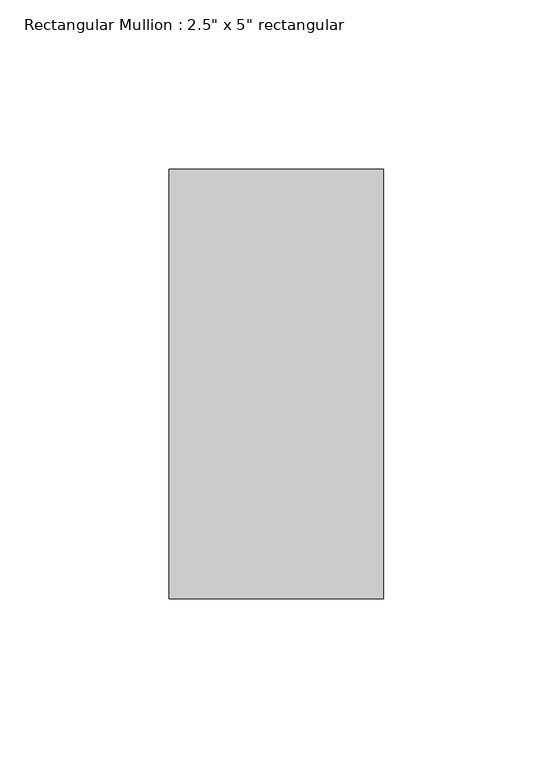
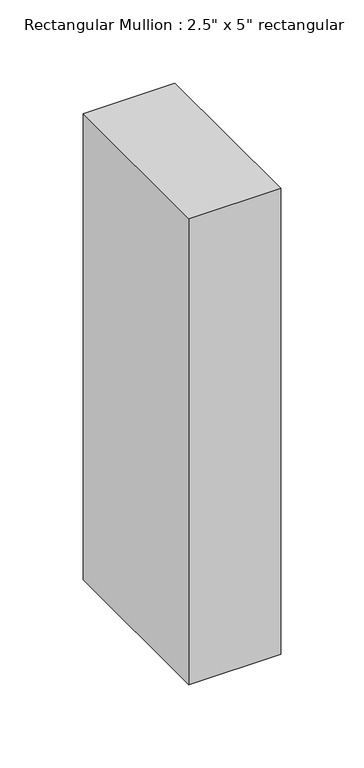
"""IFC4 building model written with IfcOpenShell, lengths in millimetres: member geometry."""

from ifc_helpers import new_model, si_unit, frame, origin, place, context, project, spatial, polyline, outline, extrude, source, transform, mapped, element, save


def member_658e374b(model_context):
    return source(origin(), model_context, "Body", "SweptSolid", [
        extrude(outline(polyline([(31.75, 63.5), (31.75, -63.5), (-31.75, -63.5), (-31.75, 63.5), (31.75, 63.5)])), frame((0.0, 0.0, -341.8283762), z_axis=(0.0, 0.0, 1.0), x_axis=(1.0, 0.0, 0.0)), (0.0, 0.0, 1.0), 341.8283762),
    ])


if __name__ == "__main__":
    model = new_model("IFC4")
    model_context = context("Model", 3, world=origin())
    ifc_project = project(units=[si_unit("LENGTHUNIT", "METRE", prefix="MILLI")], contexts=[model_context])
    site = spatial("IfcSite", under=ifc_project)
    building = spatial("IfcBuilding", under=site)
    placement = place(None, origin())
    member_shape = member_658e374b(model_context)
    element("IfcMember", 1, ObjectType="Rectangular Mullion : 2.5\" x 5\" rectangular", at=placement, inside=building, context=model_context, shape_type="MappedRepresentation", body=[
        mapped(member_shape, transform((0.0, 0.0, 0.0), x_axis=(1.0, 0.0, 0.0), y_axis=(0.0, 1.0, 0.0), z_axis=(0.0, 0.0, 1.0))),
    ])
    save(model, "model.ifc")

# Revit data of these elements
# Type "Rectangular Mullion : 2.5\" x 5\" rectangular"
#   built-in parameter 1007304 = 0.416667 (stored number, unit not read)
#   built-in parameter 1007301 = 0.104167 (stored number, unit not read)
#   built-in parameter 1007300 = 0.104167 (stored number, unit not read)
# Element 1 (IfcMember, "Rectangular Mullion : 2.5\" x 5\" rectangular")
#   Materials on its faces: "Aluminum"
# Materials
#   "Aluminum": class "Metal", colour RGB 247 247 247, transparency 0, Description = "Aluminum 6061", Cost = 0
